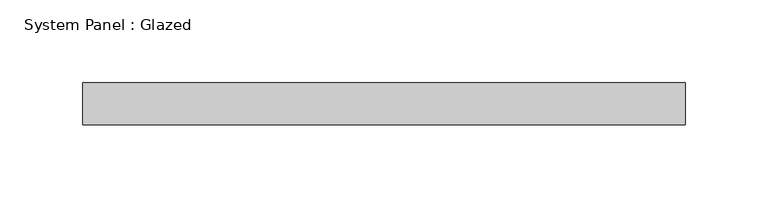
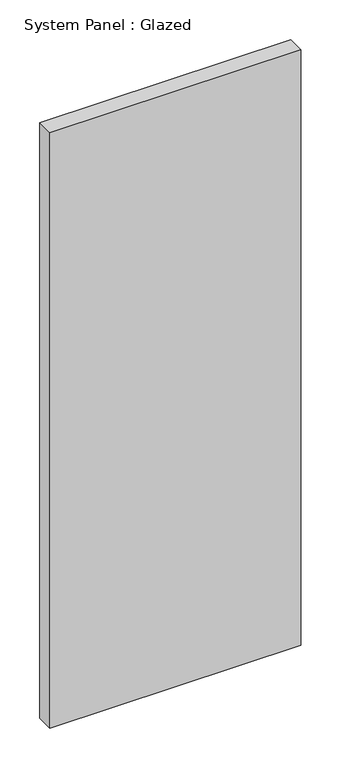
"""IFC4 building model written with IfcOpenShell, lengths in millimetres: plate geometry, System Panel : Glazed."""

from ifc_helpers import new_model, si_unit, origin, origin_with_axes, place, context, project, spatial, polyline, outline, extrude, source, transform, mapped, element, save


def system_panel_glazed_2e848b93(model_context):
    return source(origin(), model_context, "Body", "SweptSolid", [
        extrude(outline(polyline([(182.2547576, 19.05), (-182.2547576, 19.05), (-182.2547576, 44.45), (182.2547576, 44.45), (182.2547576, 19.05)])), origin_with_axes(), (0.0, 0.0, 1.0), 914.4),
    ])


if __name__ == "__main__":
    model = new_model("IFC4")
    model_context = context("Model", 3, world=origin())
    ifc_project = project(units=[si_unit("LENGTHUNIT", "METRE", prefix="MILLI")], contexts=[model_context])
    site = spatial("IfcSite", under=ifc_project)
    building = spatial("IfcBuilding", under=site)
    placement = place(None, origin())
    system_panel_glazed_shape = system_panel_glazed_2e848b93(model_context)
    element("IfcPlate", 1, ObjectType="System Panel : Glazed", at=placement, inside=building, context=model_context, shape_type="MappedRepresentation", body=[
        mapped(system_panel_glazed_shape, transform((0.0, 0.0, 0.0), x_axis=(1.0, 0.0, 0.0), y_axis=(0.0, 1.0, 0.0), z_axis=(0.0, 0.0, 1.0))),
    ])
    save(model, "model.ifc")

# Revit data of these elements
# Type "System Panel : Glazed"
#   Construction Type Id = "GSP4R"
#   Analytic Construction = "1/8 in Pilkington single glazing"
#   Visual Light Transmittance = 0.9
#   Solar Heat Gain Coefficient = 0.86
#   Heat Transfer Coefficient (U) = 1.18115 BTU/(h·ft²·°F)
# Element 1 (IfcPlate, "System Panel : Glazed")
#   Materials on its faces: "Glass"
# Materials
#   "Glass": class "Glass", colour RGB 0 128 192, transparency 0.75, Description = "Soda Lime Glass", Cost = 0
